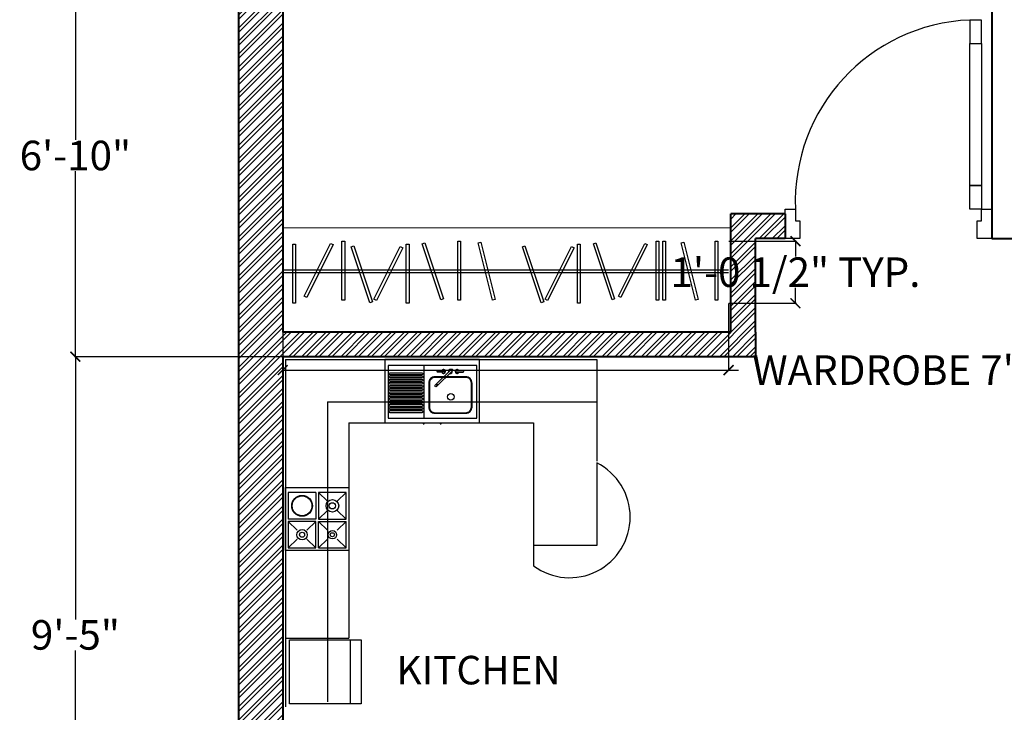
# Model space of a CAD drawing. Units: inches. Extents: x 528 to 2520, y -151 to 1354.
# Tile 16 of 41: x 1079 to 1279, y 1010 to 1151. Entities that reach past the tile are written whole.
import ezdxf

# ---------------------------------------------------------------- set-up
doc = ezdxf.new("R2010")
doc.units = ezdxf.units.IN
doc.header["$MEASUREMENT"] = 0
for name, color, linetype, lineweight in [('A-ANNO-DIMS', 2, 'Continuous', 18), ('A-AREA-IDEN', 7, 'Continuous', 18), ('A-Door', 150, 'Continuous', 25), ('A-FLOR-CASE', 11, 'Continuous', 20), ('A-WALL-PATT', 6, 'Continuous', 13), ('walls', 7, 'Continuous', 40)]:
    doc.layers.add(name, color=color, linetype=linetype, lineweight=lineweight)
for name, color, linetype in [('ESYA', 11, 'Continuous'), ('HID', 11, 'Continuous'), ('NT', 1, 'Continuous'), ('TEFRIS', 11, 'Continuous')]:
    doc.layers.add(name, color=color, linetype=linetype)
doc.styles.get("Standard").update_dxf_attribs({"font": 'arial.ttf'})
doc.dimstyles.get("Standard").update_dxf_attribs({"dimtxt": 6, "dimasz": 2, "dimexe": 0.18, "dimexo": 0.0625, "dimgap": 0.09, "dimtad": 0, "dimtih": 1, "dimtoh": 1, "dimdec": 1, "dimzin": 0, "dimdsep": 46, "dimlunit": 3, "dimtxsty": 'Standard', "dimblk": 'ARCHTICK', "dimcen": 0.09, "dimadec": 0, "dimazin": 0, "dimtfac": 1, "dimtdec": 1, "dimtofl": 0, "dimtmove": 0, "dimatfit": 3, "dimfxl": 1, "dimtolj": 1, "dimtzin": 0, "dimarcsym": 0})

# ---------------------------------------------------------------- blocks, each defined once
blk = doc.blocks.new('A$C7DB75F4D')
at = {"layer": 'A-Door'}
for points in [[(625, 740), (625, 660), (665, 660), (665, 740)], [(625, 180), (625, 660), (665, 660), (665, 180)], [(625, 100), (625, 180), (665, 180), (665, 100)], [(35, 100), (35, 60), (50, 60), (50, 50), (50, 0), (0, 0), (0, 100)], [(665, 100), (700, 100), (700, 0), (650, 0), (650, 50), (650, 60), (665, 60)]]:
    blk.add_lwpolyline(points, close=True, dxfattribs=at)
at = {"layer": 'NT'}
blk.add_arc((650, 125), 615.5, 92.3278, 182.3278, dxfattribs=at)
blk = doc.blocks.new('A$C41BE763B')
at = {"layer": 'HID'}
for p, q in [((3.395, 0.2532), (0, 0.2532)), ((3.395, 0.2332), (0, 0.2332))]:
    blk.add_line(p, q, dxfattribs=at)
for points in [[(0.0983, 0.45), (0.0983, 0), (0.0775, 0), (0.0775, 0.45)], [(0.3834, 0.447), (0.1822, 0.0445), (0.1636, 0.0538), (0.3648, 0.4563)], [(0.4716, 0.4734), (0.4716, 0.0234), (0.4508, 0.0234), (0.4508, 0.4734)], [(0.9617, 0.45), (0.9617, 0), (0.941, 0), (0.941, 0.45)], [(1.0809, 0.4606), (1.2232, 0.0337), (1.2035, 0.0271), (1.0612, 0.454)], [(1.3547, 0.4734), (1.3547, 0.0234), (1.3339, 0.0234), (1.3339, 0.4734)], [(1.5084, 0.466), (1.6175, 0.0294), (1.5974, 0.0244), (1.4882, 0.4609)], [(2.2657, 0.45), (2.2657, 0), (2.2449, 0), (2.2449, 0.45)], [(2.3849, 0.4606), (2.5272, 0.0337), (2.5075, 0.0271), (2.3652, 0.454)], [(2.7757, 0.447), (2.5745, 0.0445), (2.5559, 0.0538), (2.7572, 0.4563)], [(2.8639, 0.4734), (2.8639, 0.0234), (2.8432, 0.0234), (2.8432, 0.4734)], [(2.9139, 0.4734), (2.9139, 0.0234), (2.8932, 0.0234), (2.8932, 0.4734)], [(3.0533, 0.466), (3.1624, 0.0294), (3.1423, 0.0244), (3.0332, 0.4609)], [(3.3139, 0.4734), (3.3139, 0.0234), (3.2932, 0.0234), (3.2932, 0.4734)], [(0.5408, 0.4372), (0.6831, 0.0103), (0.6634, 0.0037), (0.5211, 0.4306)], [(0.914, 0.4236), (0.7128, 0.0211), (0.6942, 0.0304), (0.8954, 0.4329)], [(1.8448, 0.4372), (1.9871, 0.0103), (1.9674, 0.0037), (1.8251, 0.4306)], [(2.218, 0.4236), (2.0167, 0.0211), (1.9981, 0.0304), (2.1994, 0.4329)]]:
    blk.add_lwpolyline(points, close=True, dxfattribs=at)
blk = doc.blocks.new('AR365L')
blk.add_line((0, 0.0995), (0.61, 0.0995))
blk.add_lwpolyline([(0, 0), (0, 0.68), (0.61, 0.68), (0.61, 0)], close=True)
blk = doc.blocks.new('FIRIN1')
at = {"layer": 'ESYA'}
for p, q in [((0.2875, -0.05), (0.2875, -0.3006)), ((0.3983, -0.1319), (0.3125, -0.05)), ((0.575, -0.05), (0.4892, -0.1319)), ((0.3983, -0.2187), (0.3125, -0.3006)), ((0.575, -0.3006), (0.4892, -0.2187)), ((0.2875, -0.3006), (0.025, -0.3006)), ((0.025, -0.3244), (0.1108, -0.4063)), ((0.2017, -0.4063), (0.2875, -0.3244)), ((0.3983, -0.4063), (0.3125, -0.3244)), ((0.575, -0.3244), (0.4892, -0.4063)), ((0.025, -0.575), (0.1108, -0.4931)), ((0.2017, -0.4931), (0.2875, -0.575)), ((0.3983, -0.4931), (0.3125, -0.575)), ((0.575, -0.575), (0.4892, -0.4931))]:
    blk.add_line(p, q, dxfattribs=at)
blk.add_lwpolyline([(0, 0), (0.6, 0), (0.6, -0.6), (0, -0.6)], close=True, dxfattribs=at)
for points in [[(0.2875, -0.05), (0.025, -0.05), (0.025, -0.3006)], [(0.3125, -0.05), (0.3125, -0.3006), (0.575, -0.3006)], [(0.575, -0.3006), (0.575, -0.05), (0.3125, -0.05)], [(0.2875, -0.575), (0.2875, -0.3244), (0.025, -0.3244)], [(0.025, -0.3244), (0.025, -0.575)], [(0.3125, -0.575), (0.3125, -0.3244), (0.575, -0.3244)], [(0.3125, -0.575), (0.575, -0.575), (0.575, -0.3244)], [(0.025, -0.575), (0.2875, -0.575)]]:
    blk.add_lwpolyline(points, dxfattribs=at)
for centre, radius in [((0.1562, -0.1753), 0.0986), ((0.1562, -0.1753), 0.0936), ((0.4438, -0.1753), 0.0597), ((0.4438, -0.1753), 0.0294), ((0.1562, -0.4497), 0.0492), ((0.1562, -0.4497), 0.0242), ((0.4438, -0.4497), 0.0398), ((0.4438, -0.4497), 0.0196)]:
    blk.add_circle(centre, radius, dxfattribs=at)
blk = doc.blocks.new('ncvn')
for p, q in [((77868.38, -4466.7), (77868.38, -4520.7)), ((77949.38, -4466.7), (77868.38, -4466.7)), ((77949.38, -4520.7), (77949.38, -4466.7))]:
    blk.add_line(p, q)
at = {"layer": 'TEFRIS'}
for p, q in [((77783.66, -4466.69), (77783.66, -4763.38)), ((77783.66, -4466.69), (78049.52, -4466.69)), ((77901.95, -4516.62), (77901.95, -4471.62)), ((78049.52, -4466.69), (78049.52, -4553.55)), ((77819.66, -4502.83), (77819.66, -4759.23)), ((77819.66, -4502.83), (78049.52, -4502.83)), ((77837.66, -4520.83), (77837.66, -4704.71)), ((77837.66, -4520.83), (77995.52, -4520.83)), ((77868.38, -4520.7), (77949.38, -4520.7)), ((77995.52, -4520.83), (77995.52, -4642.99)), ((78049.52, -4554.99), (78049.52, -4625.66)), ((78049.52, -4625.66), (77995.83, -4625.66)), ((77783.66, -4704.71), (77837.66, -4704.71))]:
    blk.add_line(p, q, dxfattribs=at)
for points in [[(77868.38, -4466.7), (77868.38, -4520.7), (77949.38, -4520.7), (77949.38, -4466.7)], [(77871.35, -4471.62), (77871.35, -4516.62), (77946.95, -4516.62), (77946.95, -4471.62)]]:
    blk.add_lwpolyline(points, close=True, dxfattribs=at)
for points in [[(77873.15, -4477.92), (77900.15, -4477.92, -1), (77900.15, -4479.72), (77873.15, -4479.72, -1), (77873.15, -4477.92)], [(77873.15, -4480.62), (77900.15, -4480.62, -1), (77900.15, -4482.42), (77873.15, -4482.42, -1), (77873.15, -4480.62)], [(77873.15, -4483.32), (77900.15, -4483.32, -1), (77900.15, -4485.12), (77873.15, -4485.12, -1), (77873.15, -4483.32)], [(77873.15, -4486.02), (77900.15, -4486.02, -1), (77900.15, -4487.82), (77873.15, -4487.82, -1), (77873.15, -4486.02)], [(77873.15, -4488.72), (77900.15, -4488.72, -1), (77900.15, -4490.52), (77873.15, -4490.52, -1), (77873.15, -4488.72)], [(77873.15, -4491.42), (77900.15, -4491.42, -1), (77900.15, -4493.22), (77873.15, -4493.22, -1), (77873.15, -4491.42)], [(77873.15, -4494.12), (77900.15, -4494.12, -1), (77900.15, -4495.92), (77873.15, -4495.92, -1), (77873.15, -4494.12)], [(77873.15, -4496.82), (77900.15, -4496.82, -1), (77900.15, -4498.62), (77873.15, -4498.62, -1), (77873.15, -4496.82)], [(77873.15, -4499.52), (77900.15, -4499.52, -1), (77900.15, -4501.32), (77873.15, -4501.32, -1), (77873.15, -4499.52)], [(77873.15, -4502.22), (77900.15, -4502.22, -1), (77900.15, -4504.02), (77873.15, -4504.02, -1), (77873.15, -4502.22)], [(77873.15, -4504.92), (77900.15, -4504.92, -1), (77900.15, -4506.72), (77873.15, -4506.72, -1), (77873.15, -4504.92)], [(77873.15, -4507.62), (77900.15, -4507.62, -1), (77900.15, -4509.42), (77873.15, -4509.42, -1), (77873.15, -4507.62)], [(77873.15, -4510.32), (77900.15, -4510.32, -1), (77900.15, -4512.12), (77873.15, -4512.12, -1), (77873.15, -4510.32)]]:
    blk.add_lwpolyline(points, format="xyb", dxfattribs=at)
for points in [[(77905.95, -4486.73), (77905.95, -4507.22, 0.414214), (77911.35, -4512.62), (77937.55, -4512.62, 0.414214), (77942.95, -4507.22), (77942.95, -4486.73, 0.414214), (77937.55, -4481.33), (77911.35, -4481.33, 0.414214)], [(77911.5, -4488.58), (77925.04, -4475.05, -1), (77926.25, -4476.26), (77912.72, -4489.8, -1)], [(77913.54, -4476.29), (77919.71, -4476.29, -0.563183), (77919.71, -4477.44), (77913.54, -4477.44, -1)], [(77935.33, -4476.29), (77929.17, -4476.29, 0.563183), (77929.17, -4477.44), (77935.33, -4477.44, 1)], [(77906.49, -4486.73), (77906.49, -4507.22, 0.414214), (77911.35, -4512.08), (77937.55, -4512.08, 0.414214), (77942.41, -4507.22), (77942.41, -4486.73, 0.414214), (77937.55, -4481.87), (77911.35, -4481.87, 0.414214)]]:
    blk.add_lwpolyline(points, format="xyb", close=True, dxfattribs=at)
for points in [[(77901.23, -4520.7), (77901.23, -4521.6), (77902.13, -4521.6), (77902.13, -4520.7)], [(77915.63, -4520.7), (77915.63, -4521.6), (77916.53, -4521.6), (77916.53, -4520.7)]]:
    blk.add_lwpolyline(points, dxfattribs=at)
for centre, radius in [((77913.01, -4488.3), 0.571), ((77924.89, -4498.48), 2.86)]:
    blk.add_circle(centre, radius, dxfattribs=at)
for centre, radius, start, end in [((77918.69, -4476.87), 1.71, 199.47122, 160.52878), ((77924.44, -4476.87), 1.71, 75, 195), ((77924.44, -4476.87), 1.71, 255, 15), ((77930.19, -4476.87), 1.71, 19.47122, 340.52878), ((78026.22, -4601.26), 51.8, 233.6588, 63.26709)]:
    blk.add_arc(centre, radius, start, end, dxfattribs=at)
at = {"layer": 'TEFRIS', "xscale": 90, "yscale": 90, "zscale": 90}
blk.add_blockref('FIRIN1', (77783.76, -4575.88), dxfattribs=at)
at = {"layer": 'TEFRIS', "xscale": 90, "yscale": 90, "zscale": 90, "rotation": 90}
blk.add_blockref('AR365L', (77848.22, -4760.91), dxfattribs=at)
blk = doc.blocks.new('_ArchTick')
at = {"color": 0, "linetype": 'ByBlock', "const_width": 0.15}
blk.add_lwpolyline([(-0.5, -0.5), (0.5, 0.5)], dxfattribs=at)
blk = doc.blocks.new('*D58')
at = {"layer": 'A-ANNO-DIMS', "color": 0, "lineweight": -2, "transparency": 16777216}
for p, q in [((1132.88, 1092.9), (1132.88, 1079.21)), ((1223.4, 1092.9), (1223.4, 1079.21)), ((1132.88, 1079.39), (1223.4, 1079.39)), ((1223.4, 1079.39), (1225.4, 1079.39))]:
    blk.add_line(p, q, dxfattribs=at)
at = {"layer": 'Defpoints', "color": 0, "transparency": 16777216}
for p in [(1132.88, 1092.96), (1223.4, 1092.96), (1223.4, 1079.39)]:
    blk.add_point(p, dxfattribs=at)
at = {"layer": 'A-ANNO-DIMS', "color": 0, "lineweight": -2, "transparency": 16777216, "xscale": 2, "yscale": 2, "zscale": 2, "rotation": 180}
blk.add_blockref('_ArchTick', (1132.88, 1079.39), dxfattribs=at)
at = {"layer": 'A-ANNO-DIMS', "color": 0, "lineweight": -2, "transparency": 16777216, "xscale": 2, "yscale": 2, "zscale": 2}
blk.add_blockref('_ArchTick', (1223.4, 1079.39), dxfattribs=at)
at = {"layer": 'A-ANNO-DIMS', "color": 0, "transparency": 16777216, "insert": (1276.74, 1079.39), "char_height": 6, "attachment_point": 5}
blk.add_mtext('\\A1;WARDROBE 7\'-6 1/2" TYP.', dxfattribs=at)
blk = doc.blocks.new('*D59')
at = {"layer": 'A-ANNO-DIMS', "color": 0, "lineweight": -2, "transparency": 16777216}
for p, q in [((1223.46, 1105.59), (1237.16, 1105.59)), ((1236.98, 1105.59), (1236.98, 1102.47)), ((1236.98, 1092.96), (1236.98, 1096.08)), ((1223.46, 1092.96), (1237.16, 1092.96))]:
    blk.add_line(p, q, dxfattribs=at)
at = {"layer": 'Defpoints', "color": 0, "transparency": 16777216}
for p in [(1223.4, 1105.59), (1236.98, 1105.59), (1223.4, 1092.96)]:
    blk.add_point(p, dxfattribs=at)
at = {"layer": 'A-ANNO-DIMS', "color": 0, "lineweight": -2, "transparency": 16777216, "xscale": 2, "yscale": 2, "zscale": 2}
for p, rotation in [((1236.98, 1105.59), 90), ((1236.98, 1092.96), 270)]:
    blk.add_blockref('_ArchTick', p, dxfattribs=dict(at, rotation=rotation))
at = {"layer": 'A-ANNO-DIMS', "color": 0, "transparency": 16777216, "insert": (1236.98, 1099.28), "char_height": 6, "attachment_point": 5}
blk.add_mtext('\\A1;1\'-0 1/2" TYP.', dxfattribs=at)
blk = doc.blocks.new('*D97')
at = {"layer": 'A-ANNO-DIMS', "color": 0, "lineweight": -2, "transparency": 16777216}
for p, q in [((1132.82, 1082.1), (1090.6, 1082.1)), ((1090.78, 1082.1), (1090.78, 1028.76)), ((1090.78, 969.1), (1090.78, 1022.45)), ((1123.82, 969.1), (1090.6, 969.1))]:
    blk.add_line(p, q, dxfattribs=at)
at = {"layer": 'Defpoints', "color": 0, "transparency": 16777216}
for p in [(1090.78, 1082.1), (1132.88, 1082.1), (1123.88, 969.1)]:
    blk.add_point(p, dxfattribs=at)
at = {"layer": 'A-ANNO-DIMS', "color": 0, "lineweight": -2, "transparency": 16777216, "xscale": 2, "yscale": 2, "zscale": 2}
for p, rotation in [((1090.78, 1082.1), 90), ((1090.78, 969.1), 270)]:
    blk.add_blockref('_ArchTick', p, dxfattribs=dict(at, rotation=rotation))
at = {"layer": 'A-ANNO-DIMS', "color": 0, "transparency": 16777216, "insert": (1090.78, 1025.6), "char_height": 6, "attachment_point": 5}
blk.add_mtext('\\A1;9\'-5"', dxfattribs=at)
blk = doc.blocks.new('*D99')
at = {"layer": 'A-ANNO-DIMS', "color": 0, "lineweight": -2, "transparency": 16777216}
for p, q in [((1132.82, 1163.86), (1090.6, 1163.86)), ((1090.78, 1163.86), (1090.78, 1126.13)), ((1090.78, 1082.1), (1090.78, 1119.83)), ((1132.82, 1082.1), (1090.6, 1082.1))]:
    blk.add_line(p, q, dxfattribs=at)
at = {"layer": 'Defpoints', "color": 0, "transparency": 16777216}
for p in [(1132.88, 1163.86), (1090.78, 1082.1), (1132.88, 1082.1)]:
    blk.add_point(p, dxfattribs=at)
at = {"layer": 'A-ANNO-DIMS', "color": 0, "lineweight": -2, "transparency": 16777216, "xscale": 2, "yscale": 2, "zscale": 2}
for p, rotation in [((1090.78, 1163.86), 90), ((1090.78, 1082.1), 270)]:
    blk.add_blockref('_ArchTick', p, dxfattribs=dict(at, rotation=rotation))
at = {"layer": 'A-ANNO-DIMS', "color": 0, "transparency": 16777216, "insert": (1090.78, 1122.98), "char_height": 6, "attachment_point": 5}
blk.add_mtext('\\A1;6\'-10"', dxfattribs=at)

msp = doc.modelspace()

# ---------------------------------------------------------------- hatches: boundary and pattern name
at = {"layer": 'A-WALL-PATT'}
h = msp.add_hatch(dxfattribs=at)
h.set_pattern_fill('ANSI32', color=256, scale=5)
h.set_pattern_definition([(45, (537.1868, 0), (-1.3258252, 1.3258252), []), (45, (538.0707, 0), (-1.3258252, 1.3258252), [])])
h.paths.add_polyline_path([(1132.88, 1163.86), (1123.88, 1163.86), (1123.88, 969.1), (1135.43, 969.1), (1140.43, 969.1), (1140.43, 974.1), (1132.88, 974.1), (1132.88, 1082.1), (1228.88, 1082.1), (1228.88, 1087.1), (1228.88, 1106.1), (1234.88, 1106.1), (1234.88, 1111.1), (1223.88, 1111.1), (1223.88, 1087.1), (1132.88, 1087.1)])
h.paths.add_polyline_path([(1225.89, 974.1), (1188.43, 974.1), (1188.43, 969.1), (1225.89, 969.1)])
h.paths.add_polyline_path([(1422.88, 1171.37), (1413.88, 1171.37), (1413.88, 1111.1), (1323.88, 1111.1), (1323.88, 1106.1), (1413.88, 1106.1), (1413.88, 974.1), (1323.88, 974.1), (1323.88, 969.1), (1413.88, 969.1), (1413.88, 825.1), (1371.88, 825.1), (1371.88, 816.1), (1422.88, 816.1)])
h.paths.add_polyline_path([(1422.88, 1317.1), (1413.84, 1317.1), (1413.84, 1308.1), (1413.88, 1308.1), (1413.88, 1248.1), (1359.88, 1248.1), (1359.88, 1243.1), (1413.88, 1243.1), (1413.88, 1219.37), (1422.88, 1219.37)])
h.paths.add_polyline_path([(1389.84, 1317.1), (1324.88, 1317.1), (1324.88, 1248.1), (1321.45, 1248.1), (1321.45, 1243.1), (1329.88, 1243.1), (1329.88, 1249.1), (1329.88, 1308.1), (1389.84, 1308.1)])
h.paths.add_polyline_path([(1221.88, 1317.1), (1156.88, 1317.1), (1156.88, 1308.1), (1216.88, 1308.1), (1216.88, 1248.1), (1216.88, 1243.1), (1221.88, 1243.1), (1221.88, 1248.25)])
h.paths.add_polyline_path([(1132.88, 1308.1), (1132.88, 1317.1), (1123.88, 1317.1), (1123.88, 1211.86), (1132.88, 1211.86), (1132.88, 1243.1), (1186.88, 1243.1), (1186.88, 1248.1), (1132.88, 1248.1)])
h.paths.add_polyline_path([(1281.88, 969.1), (1281.88, 974.1), (1261.89, 974.1), (1261.89, 969.1), (1276.88, 969.1), (1276.88, 874.29), (1281.88, 874.29)])
h.paths.add_polyline_path([(1276.88, 969.1), (1264.88, 969.1), (1264.88, 965.12), (1267.92, 965.12), (1267.92, 961.68), (1271.62, 961.68), (1271.62, 957.24), (1276.88, 957.24)], flags=17)
h.paths.add_polyline_path([(1323.88, 825.1), (1281.88, 825.1), (1281.88, 832.29), (1276.88, 832.29), (1276.88, 816.1), (1323.88, 816.1)])

# ---------------------------------------------------------------- linework, layer by layer
at = {"layer": 'A-FLOR-CASE'}
msp.add_line((1132.88, 1108.27), (1223.88, 1108.27), dxfattribs=at)
at = {"layer": 'walls'}
for p, q in [((1123.88, 1317.1), (1123.88, 969.1)), ((1132.88, 1243.1), (1132.88, 1087.1)), ((1276.88, 1243.1), (1276.88, 1111.1)), ((1223.88, 1087.1), (1223.88, 1111.1)), ((1234.88, 1111.1), (1223.88, 1111.1)), ((1234.88, 1111.1), (1234.88, 1106.1)), ((1276.88, 1111.1), (1276.88, 1106.1)), ((1228.88, 1087.1), (1228.88, 1106.1)), ((1234.88, 1106.1), (1228.88, 1106.1)), ((1276.88, 1106.1), (1281.88, 1106.1)), ((1223.88, 1087.1), (1132.88, 1087.1)), ((1228.88, 1087.1), (1228.88, 1082.1)), ((1132.88, 1082.1), (1132.88, 974.1)), ((1228.88, 1082.1), (1132.88, 1082.1))]:
    msp.add_line(p, q, dxfattribs=at)

# ---------------------------------------------------------------- block references
at = {"layer": 'A-Door', "xscale": 0.0600000000000059, "yscale": 0.0600000000000059, "zscale": 0.0600000000000059}
msp.add_blockref('A$C7DB75F4D', (1234.88, 1106.1), dxfattribs=at)
at = {"layer": 'A-FLOR-CASE'}
for name, p, xscale, yscale, zscale in [('A$C41BE763B', (1132.88, 1092.96), 26.66231123505322, 26.66231123505322, 26.66231123505322), ('ncvn', (-17359.4, 2143.47), 0.2377471155606993, 0.2377471155606993, 0.2377471155606993)]:
    msp.add_blockref(name, p, dxfattribs=dict(at, xscale=xscale, yscale=yscale, zscale=zscale))

# ---------------------------------------------------------------- texts
at = {"layer": 'A-AREA-IDEN'}
msp.add_text('KITCHEN', height=5.793, dxfattribs=at).set_placement((1155.99, 1015.55))

# ---------------------------------------------------------------- dimensions: what is measured, and where the dimension line sits
at = {"layer": 'A-ANNO-DIMS'}
for p1, picture, middle in [((1132.88, 1163.86), '*D99', (1090.78, 1122.98)), ((1123.88, 969.1), '*D97', (1090.78, 1025.6))]:
    dim = msp.add_linear_dim(base=(1090.78, 1082.1), p1=p1, p2=(1132.88, 1082.1), angle=90, dimstyle='Standard', override={"dimdec": 1, "dimlfac": 1, "dimrnd": 0, "dimzin": 1, "dimdsep": 46, "dimlunit": 4, "dimfrac": 2}, dxfattribs=at)
    dim.commit()
    dim.dimension.update_dxf_attribs({"geometry": picture, "text_midpoint": middle})
dim = msp.add_linear_dim(base=(1236.98, 1105.59), p1=(1223.4, 1092.96), p2=(1223.4, 1105.59), angle=90, text='<> TYP.', dimstyle='Standard', override={"dimdec": 1, "dimlfac": 1, "dimrnd": 0, "dimzin": 1, "dimdsep": 46, "dimlunit": 4, "dimfrac": 2}, dxfattribs=at)
dim.commit()
dim.dimension.update_dxf_attribs({"geometry": '*D59', "text_midpoint": (1236.98, 1099.28)})
dim = msp.add_linear_dim(base=(1223.4, 1079.39), p1=(1132.88, 1092.96), p2=(1223.4, 1092.96), text='WARDROBE <> TYP.', dimstyle='Standard', override={"dimdec": 1, "dimlfac": 1, "dimrnd": 0, "dimzin": 1, "dimdsep": 46, "dimlunit": 4, "dimfrac": 2}, dxfattribs=at)
dim.commit()
dim.dimension.update_dxf_attribs({"geometry": '*D58', "text_midpoint": (1276.74, 1079.39)})

doc.saveas('drawing.dxf')
